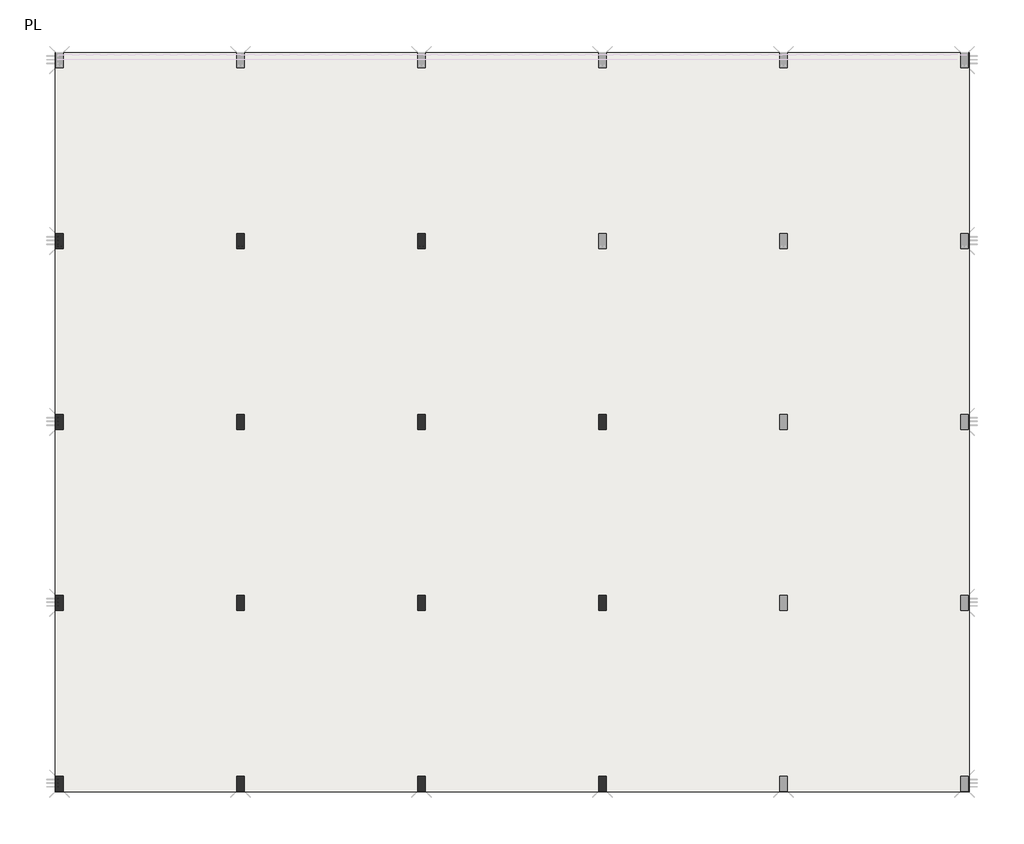
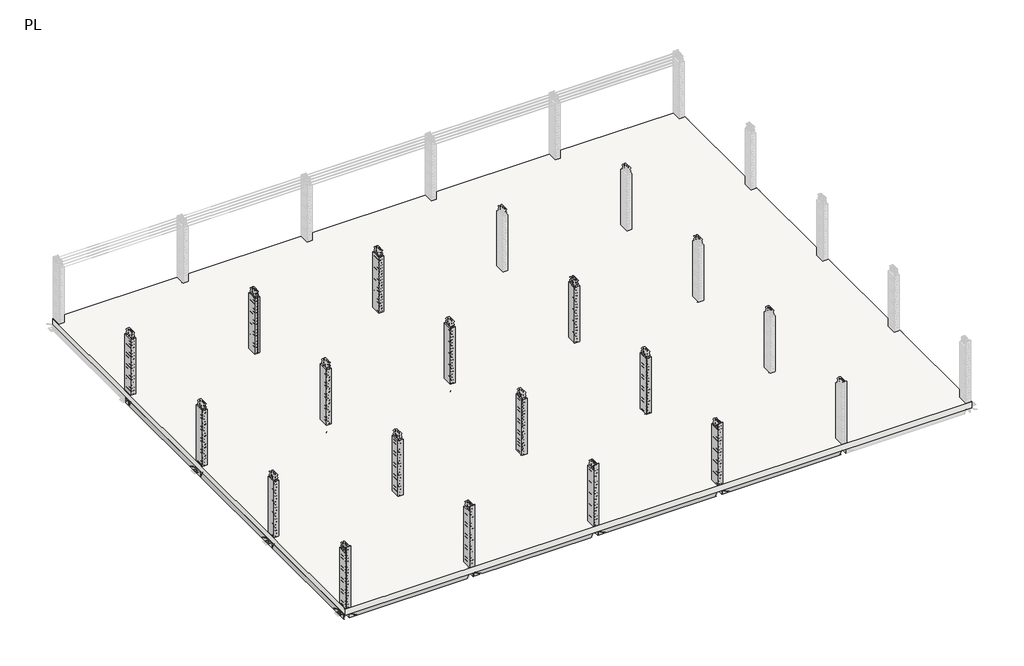
# One storey, part 1 of 10: 25 beams, 15 columns, 1 slab.
"""IFC4 building model written with IfcOpenShell, lengths in millimetres."""

from ifc_helpers import new_model, si_unit, frame, origin, place, context, project, spatial, polyline, outline, extrude, faceted_brep, element, save

model = new_model("IFC4")

# Units and contexts
model_context = context("Model", 3, world=origin())
ifc_project = project(units=[si_unit("LENGTHUNIT", "METRE", prefix="MILLI")], contexts=[model_context])

# Site, building, storey
site = spatial("IfcSite", under=ifc_project)
building = spatial("IfcBuilding", under=site)
storey = spatial("IfcBuildingStorey", under=building, Name="PL", Elevation=271.0)

# Beams
placement = place(None, origin())
element("IfcBeam", 1, ObjectType="Concrete-Rectangular Beam : 300 x 600mm", at=placement, inside=storey, context=model_context, shape_type="Brep", body=[
    faceted_brep([(-16585.9544379, -20429.1167521, -329.0), (-16560.9544379, -20429.1167521, -329.0), (-16560.9544379, -20429.1167521, -29.0), (-16585.9544379, -20429.1167521, -29.0), (-16560.9544379, -20129.1167521, -329.0), (-16585.9544379, -20129.1167521, -329.0), (-16585.9544379, -20129.1167521, -29.0), (-16560.9544379, -20129.1167521, -29.0)], [[[0, 1, 2, 3]], [[4, 1, 0, 5]], [[4, 5, 6, 7]], [[1, 4, 7, 2]], [[5, 0, 3, 6]], [[3, 2, 7, 6]]]),
    faceted_brep([(-22956.9544379, -20129.1167521, -329.0), (-22956.9544379, -20429.1167521, -329.0), (-22956.9544379, -20429.1167521, -29.0), (-22956.9544379, -20129.1167521, -29.0), (-22931.9544379, -20429.1167521, -329.0), (-22931.9544379, -20129.1167521, -329.0), (-22931.9544379, -20129.1167521, -29.0), (-22931.9544379, -20429.1167521, -29.0)], [[[0, 1, 2, 3]], [[4, 5, 6, 7]], [[1, 4, 7, 2]], [[1, 0, 5, 4]], [[5, 0, 3, 6]], [[3, 2, 7, 6]]]),
    faceted_brep([(-22681.9544379, -20129.1167521, -329.0), (-22681.9544379, -20429.1167521, -329.0), (-22681.9544379, -20429.1167521, -29.0), (-22681.9544379, -20129.1167521, -29.0), (-16835.9544379, -20429.1167521, -329.0), (-16835.9544379, -20129.1167521, -329.0), (-16835.9544379, -20129.1167521, -29.0), (-16835.9544379, -20429.1167521, -29.0), (-22656.9544379, -20129.1167521, -329.0), (-16860.9544379, -20129.1167521, -329.0), (-22656.9544379, -20129.1167521, -29.0), (-16860.9544379, -20129.1167521, -29.0)], [[[0, 1, 2, 3]], [[4, 5, 6, 7]], [[1, 4, 7, 2]], [[1, 0, 8, 9, 5, 4]], [[5, 9, 8, 0, 3, 10, 11, 6]], [[3, 2, 7, 6, 11, 10]]]),
])
element("IfcBeam", 2, ObjectType="Concrete-Rectangular Beam : 300 x 600mm", at=placement, inside=storey, context=model_context, shape_type="Brep", body=[
    faceted_brep([(-10489.9544379, -20429.1167521, -329.0), (-10464.9544379, -20429.1167521, -329.0), (-10464.9544379, -20429.1167521, -29.0), (-10489.9544379, -20429.1167521, -29.0), (-10464.9544379, -20129.1167521, -329.0), (-10489.9544379, -20129.1167521, -329.0), (-10489.9544379, -20129.1167521, -29.0), (-10464.9544379, -20129.1167521, -29.0)], [[[0, 1, 2, 3]], [[4, 1, 0, 5]], [[4, 5, 6, 7]], [[1, 4, 7, 2]], [[5, 0, 3, 6]], [[3, 2, 7, 6]]]),
    faceted_brep([(-16560.9544379, -20129.1167521, -329.0), (-16560.9544379, -20429.1167521, -329.0), (-16560.9544379, -20429.1167521, -29.0), (-16560.9544379, -20129.1167521, -29.0), (-10739.9544379, -20429.1167521, -329.0), (-10739.9544379, -20129.1167521, -329.0), (-10739.9544379, -20129.1167521, -29.0), (-10739.9544379, -20429.1167521, -29.0), (-10764.9544379, -20129.1167521, -329.0), (-10764.9544379, -20129.1167521, -29.0)], [[[0, 1, 2, 3]], [[4, 5, 6, 7]], [[1, 4, 7, 2]], [[1, 0, 8, 5, 4]], [[5, 8, 0, 3, 9, 6]], [[3, 2, 7, 6, 9]]]),
])
element("IfcBeam", 3, ObjectType="Concrete-Rectangular Beam : 300 x 600mm", at=placement, inside=storey, context=model_context, shape_type="Brep", body=[
    faceted_brep([(-4393.9544379, -20429.1167521, -329.0), (-4368.9544379, -20429.1167521, -329.0), (-4368.9544379, -20429.1167521, -29.0), (-4393.9544379, -20429.1167521, -29.0), (-4368.9544379, -20129.1167521, -329.0), (-4393.9544379, -20129.1167521, -329.0), (-4393.9544379, -20129.1167521, -29.0), (-4368.9544379, -20129.1167521, -29.0)], [[[0, 1, 2, 3]], [[4, 1, 0, 5]], [[4, 5, 6, 7]], [[1, 4, 7, 2]], [[5, 0, 3, 6]], [[3, 2, 7, 6]]]),
    faceted_brep([(-10464.9544379, -20129.1167521, -329.0), (-10464.9544379, -20429.1167521, -329.0), (-10464.9544379, -20429.1167521, -29.0), (-10464.9544379, -20129.1167521, -29.0), (-4643.9544379, -20429.1167521, -329.0), (-4643.9544379, -20129.1167521, -329.0), (-4643.9544379, -20129.1167521, -29.0), (-4643.9544379, -20429.1167521, -29.0), (-4668.9544379, -20129.1167521, -329.0), (-4668.9544379, -20129.1167521, -29.0)], [[[0, 1, 2, 3]], [[4, 5, 6, 7]], [[1, 4, 7, 2]], [[1, 0, 8, 5, 4]], [[5, 8, 0, 3, 9, 6]], [[3, 2, 7, 6, 9]]]),
])
element("IfcBeam", 4, ObjectType="Concrete-Rectangular Beam : 300 x 600mm", at=placement, inside=storey, context=model_context, shape_type="Brep", body=[
    faceted_brep([(1702.0455621, -20429.1167521, -329.0), (1727.0455621, -20429.1167521, -329.0), (1727.0455621, -20429.1167521, -29.0), (1702.0455621, -20429.1167521, -29.0), (1727.0455621, -20129.1167521, -329.0), (1702.0455621, -20129.1167521, -329.0), (1702.0455621, -20129.1167521, -29.0), (1727.0455621, -20129.1167521, -29.0)], [[[0, 1, 2, 3]], [[4, 1, 0, 5]], [[4, 5, 6, 7]], [[1, 4, 7, 2]], [[5, 0, 3, 6]], [[3, 2, 7, 6]]]),
    faceted_brep([(-4368.9544379, -20129.1167521, -329.0), (-4368.9544379, -20429.1167521, -329.0), (-4368.9544379, -20429.1167521, -29.0), (-4368.9544379, -20129.1167521, -29.0), (1452.0455621, -20429.1167521, -329.0), (1452.0455621, -20129.1167521, -329.0), (1452.0455621, -20129.1167521, -29.0), (1452.0455621, -20429.1167521, -29.0), (1427.0455621, -20129.1167521, -329.0), (1427.0455621, -20129.1167521, -29.0)], [[[0, 1, 2, 3]], [[4, 5, 6, 7]], [[1, 4, 7, 2]], [[1, 0, 8, 5, 4]], [[5, 8, 0, 3, 9, 6]], [[3, 2, 7, 6, 9]]]),
])
element("IfcBeam", 5, ObjectType="Concrete-Rectangular Beam : 300 x 600mm", at=placement, inside=storey, context=model_context, shape_type="Brep", body=[
    faceted_brep([(-16585.9544379, -14333.1167521, -329.0), (-16560.9544379, -14333.1167521, -329.0), (-16560.9544379, -14333.1167521, -29.0), (-16585.9544379, -14333.1167521, -29.0), (-16560.9544379, -14033.1167521, -329.0), (-16585.9544379, -14033.1167521, -329.0), (-16585.9544379, -14033.1167521, -29.0), (-16560.9544379, -14033.1167521, -29.0)], [[[0, 1, 2, 3]], [[4, 1, 0, 5]], [[4, 5, 6, 7]], [[1, 4, 7, 2]], [[5, 0, 3, 6]], [[3, 2, 7, 6]]]),
    faceted_brep([(-22956.9544379, -14033.1167521, -329.0), (-22956.9544379, -14333.1167521, -329.0), (-22956.9544379, -14333.1167521, -29.0), (-22956.9544379, -14033.1167521, -29.0), (-22931.9544379, -14333.1167521, -329.0), (-22931.9544379, -14033.1167521, -329.0), (-22931.9544379, -14033.1167521, -29.0), (-22931.9544379, -14333.1167521, -29.0)], [[[0, 1, 2, 3]], [[4, 5, 6, 7]], [[1, 4, 7, 2]], [[1, 0, 5, 4]], [[5, 0, 3, 6]], [[3, 2, 7, 6]]]),
    faceted_brep([(-22681.9544379, -14033.1167521, -329.0), (-22681.9544379, -14333.1167521, -329.0), (-22681.9544379, -14333.1167521, -29.0), (-22681.9544379, -14033.1167521, -29.0), (-16835.9544379, -14333.1167521, -329.0), (-16835.9544379, -14033.1167521, -329.0), (-16835.9544379, -14033.1167521, -29.0), (-16835.9544379, -14333.1167521, -29.0), (-22656.9544379, -14333.1167521, -329.0), (-16860.9544379, -14333.1167521, -329.0), (-16860.9544379, -14333.1167521, -29.0), (-22656.9544379, -14333.1167521, -29.0), (-22656.9544379, -14033.1167521, -329.0), (-16860.9544379, -14033.1167521, -329.0), (-22656.9544379, -14033.1167521, -29.0), (-16860.9544379, -14033.1167521, -29.0)], [[[0, 1, 2, 3]], [[4, 5, 6, 7]], [[1, 8, 9, 4, 7, 10, 11, 2]], [[1, 0, 12, 13, 5, 4, 9, 8]], [[5, 13, 12, 0, 3, 14, 15, 6]], [[3, 2, 11, 10, 7, 6, 15, 14]]]),
])
element("IfcBeam", 6, ObjectType="Concrete-Rectangular Beam : 300 x 600mm", at=placement, inside=storey, context=model_context, shape_type="Brep", body=[
    faceted_brep([(-10489.9544379, -14333.1167521, -329.0), (-10464.9544379, -14333.1167521, -329.0), (-10464.9544379, -14333.1167521, -29.0), (-10489.9544379, -14333.1167521, -29.0), (-10464.9544379, -14033.1167521, -329.0), (-10489.9544379, -14033.1167521, -329.0), (-10489.9544379, -14033.1167521, -29.0), (-10464.9544379, -14033.1167521, -29.0)], [[[0, 1, 2, 3]], [[4, 1, 0, 5]], [[4, 5, 6, 7]], [[1, 4, 7, 2]], [[5, 0, 3, 6]], [[3, 2, 7, 6]]]),
    faceted_brep([(-16560.9544379, -14033.1167521, -329.0), (-16560.9544379, -14333.1167521, -329.0), (-16560.9544379, -14333.1167521, -29.0), (-16560.9544379, -14033.1167521, -29.0), (-10739.9544379, -14333.1167521, -329.0), (-10739.9544379, -14033.1167521, -329.0), (-10739.9544379, -14033.1167521, -29.0), (-10739.9544379, -14333.1167521, -29.0), (-10764.9544379, -14333.1167521, -329.0), (-10764.9544379, -14333.1167521, -29.0), (-10764.9544379, -14033.1167521, -329.0), (-10764.9544379, -14033.1167521, -29.0)], [[[0, 1, 2, 3]], [[4, 5, 6, 7]], [[1, 8, 4, 7, 9, 2]], [[1, 0, 10, 5, 4, 8]], [[5, 10, 0, 3, 11, 6]], [[3, 2, 9, 7, 6, 11]]]),
])
element("IfcBeam", 7, ObjectType="Concrete-Rectangular Beam : 300 x 600mm", at=placement, inside=storey, context=model_context, shape_type="Brep", body=[
    faceted_brep([(-4393.9544379, -14333.1167521, -329.0), (-4368.9544379, -14333.1167521, -329.0), (-4368.9544379, -14333.1167521, -29.0), (-4393.9544379, -14333.1167521, -29.0), (-4368.9544379, -14033.1167521, -329.0), (-4393.9544379, -14033.1167521, -329.0), (-4393.9544379, -14033.1167521, -29.0), (-4368.9544379, -14033.1167521, -29.0)], [[[0, 1, 2, 3]], [[4, 1, 0, 5]], [[4, 5, 6, 7]], [[1, 4, 7, 2]], [[5, 0, 3, 6]], [[3, 2, 7, 6]]]),
    faceted_brep([(-10464.9544379, -14033.1167521, -329.0), (-10464.9544379, -14333.1167521, -329.0), (-10464.9544379, -14333.1167521, -29.0), (-10464.9544379, -14033.1167521, -29.0), (-4643.9544379, -14333.1167521, -329.0), (-4643.9544379, -14033.1167521, -329.0), (-4643.9544379, -14033.1167521, -29.0), (-4643.9544379, -14333.1167521, -29.0), (-4668.9544379, -14333.1167521, -329.0), (-4668.9544379, -14333.1167521, -29.0), (-4668.9544379, -14033.1167521, -329.0), (-4668.9544379, -14033.1167521, -29.0)], [[[0, 1, 2, 3]], [[4, 5, 6, 7]], [[1, 8, 4, 7, 9, 2]], [[1, 0, 10, 5, 4, 8]], [[5, 10, 0, 3, 11, 6]], [[3, 2, 9, 7, 6, 11]]]),
])
element("IfcBeam", 8, ObjectType="Concrete-Rectangular Beam : 300 x 600mm", at=placement, inside=storey, context=model_context, shape_type="Brep", body=[
    faceted_brep([(1702.0455621, -14333.1167521, -329.0), (1727.0455621, -14333.1167521, -329.0), (1727.0455621, -14333.1167521, -29.0), (1702.0455621, -14333.1167521, -29.0), (1727.0455621, -14033.1167521, -329.0), (1702.0455621, -14033.1167521, -329.0), (1702.0455621, -14033.1167521, -29.0), (1727.0455621, -14033.1167521, -29.0)], [[[0, 1, 2, 3]], [[4, 1, 0, 5]], [[4, 5, 6, 7]], [[1, 4, 7, 2]], [[5, 0, 3, 6]], [[3, 2, 7, 6]]]),
    faceted_brep([(-4368.9544379, -14033.1167521, -329.0), (-4368.9544379, -14333.1167521, -329.0), (-4368.9544379, -14333.1167521, -29.0), (-4368.9544379, -14033.1167521, -29.0), (1452.0455621, -14333.1167521, -329.0), (1452.0455621, -14033.1167521, -329.0), (1452.0455621, -14033.1167521, -29.0), (1452.0455621, -14333.1167521, -29.0), (1427.0455621, -14333.1167521, -329.0), (1427.0455621, -14333.1167521, -29.0), (1427.0455621, -14033.1167521, -329.0), (1427.0455621, -14033.1167521, -29.0)], [[[0, 1, 2, 3]], [[4, 5, 6, 7]], [[1, 8, 4, 7, 9, 2]], [[1, 0, 10, 5, 4, 8]], [[5, 10, 0, 3, 11, 6]], [[3, 2, 9, 7, 6, 11]]]),
])
element("IfcBeam", 9, ObjectType="Concrete-Rectangular Beam : 300 x 600mm", at=placement, inside=storey, context=model_context, shape_type="Brep", body=[
    faceted_brep([(-16585.9544379, -8237.1167521, -329.0), (-16560.9544379, -8237.1167521, -329.0), (-16560.9544379, -8237.1167521, -29.0), (-16585.9544379, -8237.1167521, -29.0), (-16560.9544379, -7937.1167521, -329.0), (-16585.9544379, -7937.1167521, -329.0), (-16585.9544379, -7937.1167521, -29.0), (-16560.9544379, -7937.1167521, -29.0)], [[[0, 1, 2, 3]], [[4, 1, 0, 5]], [[4, 5, 6, 7]], [[1, 4, 7, 2]], [[5, 0, 3, 6]], [[3, 2, 7, 6]]]),
    faceted_brep([(-22956.9544379, -7937.1167521, -329.0), (-22956.9544379, -8237.1167521, -329.0), (-22956.9544379, -8237.1167521, -29.0), (-22956.9544379, -7937.1167521, -29.0), (-22931.9544379, -8237.1167521, -329.0), (-22931.9544379, -7937.1167521, -329.0), (-22931.9544379, -7937.1167521, -29.0), (-22931.9544379, -8237.1167521, -29.0)], [[[0, 1, 2, 3]], [[4, 5, 6, 7]], [[1, 4, 7, 2]], [[1, 0, 5, 4]], [[5, 0, 3, 6]], [[3, 2, 7, 6]]]),
    faceted_brep([(-22681.9544379, -7937.1167521, -329.0), (-22681.9544379, -8237.1167521, -329.0), (-22681.9544379, -8237.1167521, -29.0), (-22681.9544379, -7937.1167521, -29.0), (-16835.9544379, -8237.1167521, -329.0), (-16835.9544379, -7937.1167521, -329.0), (-16835.9544379, -7937.1167521, -29.0), (-16835.9544379, -8237.1167521, -29.0), (-22656.9544379, -8237.1167521, -329.0), (-16860.9544379, -8237.1167521, -329.0), (-16860.9544379, -8237.1167521, -29.0), (-22656.9544379, -8237.1167521, -29.0), (-22656.9544379, -7937.1167521, -329.0), (-16860.9544379, -7937.1167521, -329.0), (-22656.9544379, -7937.1167521, -29.0), (-16860.9544379, -7937.1167521, -29.0)], [[[0, 1, 2, 3]], [[4, 5, 6, 7]], [[1, 8, 9, 4, 7, 10, 11, 2]], [[1, 0, 12, 13, 5, 4, 9, 8]], [[5, 13, 12, 0, 3, 14, 15, 6]], [[3, 2, 11, 10, 7, 6, 15, 14]]]),
])
element("IfcBeam", 10, ObjectType="Concrete-Rectangular Beam : 300 x 600mm", at=placement, inside=storey, context=model_context, shape_type="Brep", body=[
    faceted_brep([(-10489.9544379, -8237.1167521, -329.0), (-10464.9544379, -8237.1167521, -329.0), (-10464.9544379, -8237.1167521, -29.0), (-10489.9544379, -8237.1167521, -29.0), (-10464.9544379, -7937.1167521, -329.0), (-10489.9544379, -7937.1167521, -329.0), (-10489.9544379, -7937.1167521, -29.0), (-10464.9544379, -7937.1167521, -29.0)], [[[0, 1, 2, 3]], [[4, 1, 0, 5]], [[4, 5, 6, 7]], [[1, 4, 7, 2]], [[5, 0, 3, 6]], [[3, 2, 7, 6]]]),
    faceted_brep([(-16560.9544379, -7937.1167521, -329.0), (-16560.9544379, -8237.1167521, -329.0), (-16560.9544379, -8237.1167521, -29.0), (-16560.9544379, -7937.1167521, -29.0), (-10739.9544379, -8237.1167521, -329.0), (-10739.9544379, -7937.1167521, -329.0), (-10739.9544379, -7937.1167521, -29.0), (-10739.9544379, -8237.1167521, -29.0), (-10764.9544379, -8237.1167521, -329.0), (-10764.9544379, -8237.1167521, -29.0), (-10764.9544379, -7937.1167521, -329.0), (-10764.9544379, -7937.1167521, -29.0)], [[[0, 1, 2, 3]], [[4, 5, 6, 7]], [[1, 8, 4, 7, 9, 2]], [[1, 0, 10, 5, 4, 8]], [[5, 10, 0, 3, 11, 6]], [[3, 2, 9, 7, 6, 11]]]),
])
element("IfcBeam", 11, ObjectType="Concrete-Rectangular Beam : 300 x 600mm", at=placement, inside=storey, context=model_context, shape_type="Brep", body=[
    faceted_brep([(-4393.9544379, -8237.1167521, -329.0), (-4368.9544379, -8237.1167521, -329.0), (-4368.9544379, -8237.1167521, -29.0), (-4393.9544379, -8237.1167521, -29.0), (-4368.9544379, -7937.1167521, -329.0), (-4393.9544379, -7937.1167521, -329.0), (-4393.9544379, -7937.1167521, -29.0), (-4368.9544379, -7937.1167521, -29.0)], [[[0, 1, 2, 3]], [[4, 1, 0, 5]], [[4, 5, 6, 7]], [[1, 4, 7, 2]], [[5, 0, 3, 6]], [[3, 2, 7, 6]]]),
    faceted_brep([(-10464.9544379, -7937.1167521, -329.0), (-10464.9544379, -8237.1167521, -329.0), (-10464.9544379, -8237.1167521, -29.0), (-10464.9544379, -7937.1167521, -29.0), (-4643.9544379, -8237.1167521, -329.0), (-4643.9544379, -7937.1167521, -329.0), (-4643.9544379, -7937.1167521, -29.0), (-4643.9544379, -8237.1167521, -29.0), (-4668.9544379, -8237.1167521, -329.0), (-4668.9544379, -8237.1167521, -29.0), (-4668.9544379, -7937.1167521, -329.0), (-4668.9544379, -7937.1167521, -29.0)], [[[0, 1, 2, 3]], [[4, 5, 6, 7]], [[1, 8, 4, 7, 9, 2]], [[1, 0, 10, 5, 4, 8]], [[5, 10, 0, 3, 11, 6]], [[3, 2, 9, 7, 6, 11]]]),
])
element("IfcBeam", 12, ObjectType="Concrete-Rectangular Beam : 300 x 600mm", at=placement, inside=storey, context=model_context, shape_type="Brep", body=[
    faceted_brep([(1702.0455621, -8237.1167521, -329.0), (1727.0455621, -8237.1167521, -329.0), (1727.0455621, -8237.1167521, -29.0), (1702.0455621, -8237.1167521, -29.0), (1727.0455621, -7937.1167521, -329.0), (1702.0455621, -7937.1167521, -329.0), (1702.0455621, -7937.1167521, -29.0), (1727.0455621, -7937.1167521, -29.0)], [[[0, 1, 2, 3]], [[4, 1, 0, 5]], [[4, 5, 6, 7]], [[1, 4, 7, 2]], [[5, 0, 3, 6]], [[3, 2, 7, 6]]]),
    faceted_brep([(-4368.9544379, -7937.1167521, -329.0), (-4368.9544379, -8237.1167521, -329.0), (-4368.9544379, -8237.1167521, -29.0), (-4368.9544379, -7937.1167521, -29.0), (1452.0455621, -8237.1167521, -329.0), (1452.0455621, -7937.1167521, -329.0), (1452.0455621, -7937.1167521, -29.0), (1452.0455621, -8237.1167521, -29.0), (1427.0455621, -8237.1167521, -329.0), (1427.0455621, -8237.1167521, -29.0), (1427.0455621, -7937.1167521, -329.0), (1427.0455621, -7937.1167521, -29.0)], [[[0, 1, 2, 3]], [[4, 5, 6, 7]], [[1, 8, 4, 7, 9, 2]], [[1, 0, 10, 5, 4, 8]], [[5, 10, 0, 3, 11, 6]], [[3, 2, 9, 7, 6, 11]]]),
])
element("IfcBeam", 13, ObjectType="Concrete-Rectangular Beam : 300 x 600mm", at=placement, inside=storey, context=model_context, shape_type="Brep", body=[
    faceted_brep([(-16585.9544379, -2141.1167521, -329.0), (-16560.9544379, -2141.1167521, -329.0), (-16560.9544379, -2141.1167521, -29.0), (-16585.9544379, -2141.1167521, -29.0), (-16560.9544379, -1841.1167521, -329.0), (-16585.9544379, -1841.1167521, -329.0), (-16585.9544379, -1841.1167521, -29.0), (-16560.9544379, -1841.1167521, -29.0)], [[[0, 1, 2, 3]], [[4, 1, 0, 5]], [[4, 5, 6, 7]], [[1, 4, 7, 2]], [[5, 0, 3, 6]], [[3, 2, 7, 6]]]),
    faceted_brep([(-22956.9544379, -1841.1167521, -329.0), (-22956.9544379, -2141.1167521, -329.0), (-22956.9544379, -2141.1167521, -29.0), (-22956.9544379, -1841.1167521, -29.0), (-22931.9544379, -2141.1167521, -329.0), (-22931.9544379, -1841.1167521, -329.0), (-22931.9544379, -1841.1167521, -29.0), (-22931.9544379, -2141.1167521, -29.0)], [[[0, 1, 2, 3]], [[4, 5, 6, 7]], [[1, 4, 7, 2]], [[1, 0, 5, 4]], [[5, 0, 3, 6]], [[3, 2, 7, 6]]]),
    faceted_brep([(-22681.9544379, -1841.1167521, -329.0), (-22681.9544379, -2141.1167521, -329.0), (-22681.9544379, -2141.1167521, -29.0), (-22681.9544379, -1841.1167521, -29.0), (-16835.9544379, -2141.1167521, -329.0), (-16835.9544379, -1841.1167521, -329.0), (-16835.9544379, -1841.1167521, -29.0), (-16835.9544379, -2141.1167521, -29.0), (-22656.9544379, -2141.1167521, -329.0), (-16860.9544379, -2141.1167521, -329.0), (-16860.9544379, -2141.1167521, -29.0), (-22656.9544379, -2141.1167521, -29.0), (-22656.9544379, -1841.1167521, -329.0), (-16860.9544379, -1841.1167521, -329.0), (-22656.9544379, -1841.1167521, -29.0), (-16860.9544379, -1841.1167521, -29.0)], [[[0, 1, 2, 3]], [[4, 5, 6, 7]], [[1, 8, 9, 4, 7, 10, 11, 2]], [[1, 0, 12, 13, 5, 4, 9, 8]], [[5, 13, 12, 0, 3, 14, 15, 6]], [[3, 2, 11, 10, 7, 6, 15, 14]]]),
])
element("IfcBeam", 14, ObjectType="Concrete-Rectangular Beam : 300 x 600mm", at=placement, inside=storey, context=model_context, shape_type="Brep", body=[
    faceted_brep([(-10489.9544379, -2141.1167521, -329.0), (-10464.9544379, -2141.1167521, -329.0), (-10464.9544379, -2141.1167521, -29.0), (-10489.9544379, -2141.1167521, -29.0), (-10464.9544379, -1841.1167521, -329.0), (-10489.9544379, -1841.1167521, -329.0), (-10489.9544379, -1841.1167521, -29.0), (-10464.9544379, -1841.1167521, -29.0)], [[[0, 1, 2, 3]], [[4, 1, 0, 5]], [[4, 5, 6, 7]], [[1, 4, 7, 2]], [[5, 0, 3, 6]], [[3, 2, 7, 6]]]),
    faceted_brep([(-16560.9544379, -1841.1167521, -329.0), (-16560.9544379, -2141.1167521, -329.0), (-16560.9544379, -2141.1167521, -29.0), (-16560.9544379, -1841.1167521, -29.0), (-10739.9544379, -2141.1167521, -329.0), (-10739.9544379, -1841.1167521, -329.0), (-10739.9544379, -1841.1167521, -29.0), (-10739.9544379, -2141.1167521, -29.0), (-10764.9544379, -2141.1167521, -329.0), (-10764.9544379, -2141.1167521, -29.0), (-10764.9544379, -1841.1167521, -329.0), (-10764.9544379, -1841.1167521, -29.0)], [[[0, 1, 2, 3]], [[4, 5, 6, 7]], [[1, 8, 4, 7, 9, 2]], [[1, 0, 10, 5, 4, 8]], [[5, 10, 0, 3, 11, 6]], [[3, 2, 9, 7, 6, 11]]]),
])
element("IfcBeam", 15, ObjectType="Concrete-Rectangular Beam : 300 x 600mm", at=placement, inside=storey, context=model_context, shape_type="SweptSolid", body=[
    extrude(outline(polyline([(-22931.9544379, -20129.1167521), (-22956.9544379, -20129.1167521), (-22956.9544379, -14333.1167521), (-22931.9544379, -14333.1167521), (-22931.9544379, -14433.1167521), (-22681.9544379, -14433.1167521), (-22681.9544379, -14333.1167521), (-22656.9544379, -14333.1167521), (-22656.9544379, -20129.1167521), (-22681.9544379, -20129.1167521), (-22681.9544379, -20029.1167521), (-22931.9544379, -20029.1167521), (-22931.9544379, -20129.1167521)])), frame((0.0, 0.0, -329.0), z_axis=(0.0, 0.0, 1.0), x_axis=(1.0, 0.0, 0.0)), (0.0, 0.0, 1.0), 300.0),
])
element("IfcBeam", 16, ObjectType="Concrete-Rectangular Beam : 300 x 600mm", at=placement, inside=storey, context=model_context, shape_type="SweptSolid", body=[
    extrude(outline(polyline([(-22931.9544379, -14033.1167521), (-22956.9544379, -14033.1167521), (-22956.9544379, -8237.1167521), (-22931.9544379, -8237.1167521), (-22931.9544379, -8337.1167521), (-22681.9544379, -8337.1167521), (-22681.9544379, -8237.1167521), (-22656.9544379, -8237.1167521), (-22656.9544379, -14033.1167521), (-22681.9544379, -14033.1167521), (-22681.9544379, -13933.1167521), (-22931.9544379, -13933.1167521), (-22931.9544379, -14033.1167521)])), frame((0.0, 0.0, -329.0), z_axis=(0.0, 0.0, 1.0), x_axis=(1.0, 0.0, 0.0)), (0.0, 0.0, 1.0), 300.0),
])
element("IfcBeam", 17, ObjectType="Concrete-Rectangular Beam : 300 x 600mm", at=placement, inside=storey, context=model_context, shape_type="SweptSolid", body=[
    extrude(outline(polyline([(-22931.9544379, -7937.1167521), (-22956.9544379, -7937.1167521), (-22956.9544379, -2141.1167521), (-22931.9544379, -2141.1167521), (-22931.9544379, -2241.1167521), (-22681.9544379, -2241.1167521), (-22681.9544379, -2141.1167521), (-22656.9544379, -2141.1167521), (-22656.9544379, -7937.1167521), (-22681.9544379, -7937.1167521), (-22681.9544379, -7837.1167521), (-22931.9544379, -7837.1167521), (-22931.9544379, -7937.1167521)])), frame((0.0, 0.0, -329.0), z_axis=(0.0, 0.0, 1.0), x_axis=(1.0, 0.0, 0.0)), (0.0, 0.0, 1.0), 300.0),
])
element("IfcBeam", 18, ObjectType="Concrete-Rectangular Beam : 300 x 600mm", at=placement, inside=storey, context=model_context, shape_type="SweptSolid", body=[
    extrude(outline(polyline([(-16835.9544379, -20129.1167521), (-16860.9544379, -20129.1167521), (-16860.9544379, -14333.1167521), (-16835.9544379, -14333.1167521), (-16835.9544379, -14433.1167521), (-16585.9544379, -14433.1167521), (-16585.9544379, -14333.1167521), (-16560.9544379, -14333.1167521), (-16560.9544379, -20129.1167521), (-16585.9544379, -20129.1167521), (-16585.9544379, -20029.1167521), (-16835.9544379, -20029.1167521), (-16835.9544379, -20129.1167521)])), frame((0.0, 0.0, -329.0), z_axis=(0.0, 0.0, 1.0), x_axis=(1.0, 0.0, 0.0)), (0.0, 0.0, 1.0), 300.0),
])
element("IfcBeam", 19, ObjectType="Concrete-Rectangular Beam : 300 x 600mm", at=placement, inside=storey, context=model_context, shape_type="SweptSolid", body=[
    extrude(outline(polyline([(-16835.9544379, -14033.1167521), (-16860.9544379, -14033.1167521), (-16860.9544379, -8237.1167521), (-16835.9544379, -8237.1167521), (-16835.9544379, -8337.1167521), (-16585.9544379, -8337.1167521), (-16585.9544379, -8237.1167521), (-16560.9544379, -8237.1167521), (-16560.9544379, -14033.1167521), (-16585.9544379, -14033.1167521), (-16585.9544379, -13933.1167521), (-16835.9544379, -13933.1167521), (-16835.9544379, -14033.1167521)])), frame((0.0, 0.0, -329.0), z_axis=(0.0, 0.0, 1.0), x_axis=(1.0, 0.0, 0.0)), (0.0, 0.0, 1.0), 300.0),
])
element("IfcBeam", 20, ObjectType="Concrete-Rectangular Beam : 300 x 600mm", at=placement, inside=storey, context=model_context, shape_type="SweptSolid", body=[
    extrude(outline(polyline([(-16835.9544379, -7937.1167521), (-16860.9544379, -7937.1167521), (-16860.9544379, -2141.1167521), (-16835.9544379, -2141.1167521), (-16835.9544379, -2241.1167521), (-16585.9544379, -2241.1167521), (-16585.9544379, -2141.1167521), (-16560.9544379, -2141.1167521), (-16560.9544379, -7937.1167521), (-16585.9544379, -7937.1167521), (-16585.9544379, -7837.1167521), (-16835.9544379, -7837.1167521), (-16835.9544379, -7937.1167521)])), frame((0.0, 0.0, -329.0), z_axis=(0.0, 0.0, 1.0), x_axis=(1.0, 0.0, 0.0)), (0.0, 0.0, 1.0), 300.0),
])
element("IfcBeam", 21, ObjectType="Concrete-Rectangular Beam : 300 x 600mm", at=placement, inside=storey, context=model_context, shape_type="SweptSolid", body=[
    extrude(outline(polyline([(-10739.9544379, -20129.1167521), (-10764.9544379, -20129.1167521), (-10764.9544379, -14333.1167521), (-10739.9544379, -14333.1167521), (-10739.9544379, -14433.1167521), (-10489.9544379, -14433.1167521), (-10489.9544379, -14333.1167521), (-10464.9544379, -14333.1167521), (-10464.9544379, -20129.1167521), (-10489.9544379, -20129.1167521), (-10489.9544379, -20029.1167521), (-10739.9544379, -20029.1167521), (-10739.9544379, -20129.1167521)])), frame((0.0, 0.0, -329.0), z_axis=(0.0, 0.0, 1.0), x_axis=(1.0, 0.0, 0.0)), (0.0, 0.0, 1.0), 300.0),
])
element("IfcBeam", 22, ObjectType="Concrete-Rectangular Beam : 300 x 600mm", at=placement, inside=storey, context=model_context, shape_type="SweptSolid", body=[
    extrude(outline(polyline([(-10739.9544379, -14033.1167521), (-10764.9544379, -14033.1167521), (-10764.9544379, -8237.1167521), (-10739.9544379, -8237.1167521), (-10739.9544379, -8337.1167521), (-10489.9544379, -8337.1167521), (-10489.9544379, -8237.1167521), (-10464.9544379, -8237.1167521), (-10464.9544379, -14033.1167521), (-10489.9544379, -14033.1167521), (-10489.9544379, -13933.1167521), (-10739.9544379, -13933.1167521), (-10739.9544379, -14033.1167521)])), frame((0.0, 0.0, -329.0), z_axis=(0.0, 0.0, 1.0), x_axis=(1.0, 0.0, 0.0)), (0.0, 0.0, 1.0), 300.0),
])
element("IfcBeam", 23, ObjectType="Concrete-Rectangular Beam : 300 x 600mm", at=placement, inside=storey, context=model_context, shape_type="SweptSolid", body=[
    extrude(outline(polyline([(-10489.9544379, -7837.1167521), (-10739.9544379, -7837.1167521), (-10739.9544379, -7937.1167521), (-10764.9544379, -7937.1167521), (-10764.9544379, -2141.1167521), (-10739.9544379, -2141.1167521), (-10739.9544379, -2241.1167521), (-10489.9544379, -2241.1167521), (-10489.9544379, -2141.1167521), (-10464.9544379, -2141.1167521), (-10464.9544379, -7937.1167521), (-10489.9544379, -7937.1167521), (-10489.9544379, -7837.1167521)])), frame((0.0, 0.0, -329.0), z_axis=(0.0, 0.0, 1.0), x_axis=(1.0, 0.0, 0.0)), (0.0, 0.0, 1.0), 300.0),
])
element("IfcBeam", 24, ObjectType="Concrete-Rectangular Beam : 300 x 600mm", at=placement, inside=storey, context=model_context, shape_type="SweptSolid", body=[
    extrude(outline(polyline([(-4643.9544379, -20129.1167521), (-4668.9544379, -20129.1167521), (-4668.9544379, -14333.1167521), (-4643.9544379, -14333.1167521), (-4643.9544379, -14433.1167521), (-4393.9544379, -14433.1167521), (-4393.9544379, -14333.1167521), (-4368.9544379, -14333.1167521), (-4368.9544379, -20129.1167521), (-4393.9544379, -20129.1167521), (-4393.9544379, -20029.1167521), (-4643.9544379, -20029.1167521), (-4643.9544379, -20129.1167521)])), frame((0.0, 0.0, -329.0), z_axis=(0.0, 0.0, 1.0), x_axis=(1.0, 0.0, 0.0)), (0.0, 0.0, 1.0), 300.0),
])
element("IfcBeam", 25, ObjectType="Concrete-Rectangular Beam : 300 x 600mm", at=placement, inside=storey, context=model_context, shape_type="SweptSolid", body=[
    extrude(outline(polyline([(-4643.9544379, -14033.1167521), (-4668.9544379, -14033.1167521), (-4668.9544379, -8237.1167521), (-4643.9544379, -8237.1167521), (-4643.9544379, -8337.1167521), (-4393.9544379, -8337.1167521), (-4393.9544379, -8237.1167521), (-4368.9544379, -8237.1167521), (-4368.9544379, -14033.1167521), (-4393.9544379, -14033.1167521), (-4393.9544379, -13933.1167521), (-4643.9544379, -13933.1167521), (-4643.9544379, -14033.1167521)])), frame((0.0, 0.0, -329.0), z_axis=(0.0, 0.0, 1.0), x_axis=(1.0, 0.0, 0.0)), (0.0, 0.0, 1.0), 300.0),
])

# Columns
element("IfcColumn", 26, ObjectType="Concrete-Rectangular-Column : 500X250", at=placement, inside=storey, context=model_context, shape_type="SweptSolid", body=[
    extrude(outline(polyline([(-20529.1167521, 271.0), (-20529.1167521, 3471.4), (-20525.9346398, 3471.4), (-20525.9346398, 3171.4), (-20029.1167521, 3171.4), (-20029.1167521, 271.0), (-20529.1167521, 271.0)])), frame((-22931.9544379, 0.0, 0.0), z_axis=(1.0, 0.0, 0.0), x_axis=(0.0, 1.0, 0.0)), (0.0, 0.0, 1.0), 250.0),
])
element("IfcColumn", 27, ObjectType="Concrete-Rectangular-Column : 500X250", at=placement, inside=storey, context=model_context, shape_type="SweptSolid", body=[
    extrude(outline(polyline([(-20529.1167521, 271.0), (-20529.1167521, 3471.4), (-20525.9346398, 3471.4), (-20525.9346398, 3171.4), (-20029.1167521, 3171.4), (-20029.1167521, 271.0), (-20529.1167521, 271.0)])), frame((-16835.9544379, 0.0, 0.0), z_axis=(1.0, 0.0, 0.0), x_axis=(0.0, 1.0, 0.0)), (0.0, 0.0, 1.0), 250.0),
])
element("IfcColumn", 28, ObjectType="Concrete-Rectangular-Column : 500X250", at=placement, inside=storey, context=model_context, shape_type="SweptSolid", body=[
    extrude(outline(polyline([(-20529.1167521, 271.0), (-20529.1167521, 3471.4), (-20525.9346398, 3471.4), (-20525.9346398, 3171.4), (-20029.1167521, 3171.4), (-20029.1167521, 271.0), (-20529.1167521, 271.0)])), frame((-10739.9544379, 0.0, 0.0), z_axis=(1.0, 0.0, 0.0), x_axis=(0.0, 1.0, 0.0)), (0.0, 0.0, 1.0), 250.0),
])
element("IfcColumn", 29, ObjectType="Concrete-Rectangular-Column : 500X250", at=placement, inside=storey, context=model_context, shape_type="SweptSolid", body=[
    extrude(outline(polyline([(-20529.1167521, 271.0), (-20529.1167521, 3471.4), (-20525.9346398, 3471.4), (-20525.9346398, 3171.4), (-20029.1167521, 3171.4), (-20029.1167521, 271.0), (-20529.1167521, 271.0)])), frame((-4643.9544379, 0.0, 0.0), z_axis=(1.0, 0.0, 0.0), x_axis=(0.0, 1.0, 0.0)), (0.0, 0.0, 1.0), 250.0),
])
element("IfcColumn", 30, ObjectType="Concrete-Rectangular-Column : 500X250", at=placement, inside=storey, context=model_context, shape_type="SweptSolid", body=[
    extrude(outline(polyline([(-22931.9544379, -13933.1167521), (-22681.9544379, -13933.1167521), (-22681.9544379, -14433.1167521), (-22931.9544379, -14433.1167521), (-22931.9544379, -13933.1167521)])), frame((0.0, 0.0, 271.0), z_axis=(0.0, 0.0, 1.0), x_axis=(1.0, 0.0, 0.0)), (0.0, 0.0, 1.0), 2900.4),
])
element("IfcColumn", 31, ObjectType="Concrete-Rectangular-Column : 500X250", at=placement, inside=storey, context=model_context, shape_type="SweptSolid", body=[
    extrude(outline(polyline([(-16835.9544379, -13933.1167521), (-16585.9544379, -13933.1167521), (-16585.9544379, -14433.1167521), (-16835.9544379, -14433.1167521), (-16835.9544379, -13933.1167521)])), frame((0.0, 0.0, 271.0), z_axis=(0.0, 0.0, 1.0), x_axis=(1.0, 0.0, 0.0)), (0.0, 0.0, 1.0), 2900.4),
])
element("IfcColumn", 32, ObjectType="Concrete-Rectangular-Column : 500X250", at=placement, inside=storey, context=model_context, shape_type="SweptSolid", body=[
    extrude(outline(polyline([(-10739.9544379, -13933.1167521), (-10489.9544379, -13933.1167521), (-10489.9544379, -14433.1167521), (-10739.9544379, -14433.1167521), (-10739.9544379, -13933.1167521)])), frame((0.0, 0.0, 271.0), z_axis=(0.0, 0.0, 1.0), x_axis=(1.0, 0.0, 0.0)), (0.0, 0.0, 1.0), 2900.4),
])
element("IfcColumn", 33, ObjectType="Concrete-Rectangular-Column : 500X250", at=placement, inside=storey, context=model_context, shape_type="SweptSolid", body=[
    extrude(outline(polyline([(-4643.9544379, -13933.1167521), (-4393.9544379, -13933.1167521), (-4393.9544379, -14433.1167521), (-4643.9544379, -14433.1167521), (-4643.9544379, -13933.1167521)])), frame((0.0, 0.0, 271.0), z_axis=(0.0, 0.0, 1.0), x_axis=(1.0, 0.0, 0.0)), (0.0, 0.0, 1.0), 2900.4),
])
element("IfcColumn", 34, ObjectType="Concrete-Rectangular-Column : 500X250", at=placement, inside=storey, context=model_context, shape_type="SweptSolid", body=[
    extrude(outline(polyline([(-22931.9544379, -7837.1167521), (-22681.9544379, -7837.1167521), (-22681.9544379, -8337.1167521), (-22931.9544379, -8337.1167521), (-22931.9544379, -7837.1167521)])), frame((0.0, 0.0, 271.0), z_axis=(0.0, 0.0, 1.0), x_axis=(1.0, 0.0, 0.0)), (0.0, 0.0, 1.0), 2900.4),
])
element("IfcColumn", 35, ObjectType="Concrete-Rectangular-Column : 500X250", at=placement, inside=storey, context=model_context, shape_type="SweptSolid", body=[
    extrude(outline(polyline([(-16835.9544379, -7837.1167521), (-16585.9544379, -7837.1167521), (-16585.9544379, -8337.1167521), (-16835.9544379, -8337.1167521), (-16835.9544379, -7837.1167521)])), frame((0.0, 0.0, 271.0), z_axis=(0.0, 0.0, 1.0), x_axis=(1.0, 0.0, 0.0)), (0.0, 0.0, 1.0), 2900.4),
])
element("IfcColumn", 36, ObjectType="Concrete-Rectangular-Column : 500X250", at=placement, inside=storey, context=model_context, shape_type="SweptSolid", body=[
    extrude(outline(polyline([(-10739.9544379, -7837.1167521), (-10489.9544379, -7837.1167521), (-10489.9544379, -8337.1167521), (-10739.9544379, -8337.1167521), (-10739.9544379, -7837.1167521)])), frame((0.0, 0.0, 271.0), z_axis=(0.0, 0.0, 1.0), x_axis=(1.0, 0.0, 0.0)), (0.0, 0.0, 1.0), 2900.4),
])
element("IfcColumn", 37, ObjectType="Concrete-Rectangular-Column : 500X250", at=placement, inside=storey, context=model_context, shape_type="SweptSolid", body=[
    extrude(outline(polyline([(-4643.9544379, -7837.1167521), (-4393.9544379, -7837.1167521), (-4393.9544379, -8337.1167521), (-4643.9544379, -8337.1167521), (-4643.9544379, -7837.1167521)])), frame((0.0, 0.0, 271.0), z_axis=(0.0, 0.0, 1.0), x_axis=(1.0, 0.0, 0.0)), (0.0, 0.0, 1.0), 2900.4),
])
element("IfcColumn", 38, ObjectType="Concrete-Rectangular-Column : 500X250", at=placement, inside=storey, context=model_context, shape_type="SweptSolid", body=[
    extrude(outline(polyline([(-22931.9544379, -1741.1167521), (-22681.9544379, -1741.1167521), (-22681.9544379, -2241.1167521), (-22931.9544379, -2241.1167521), (-22931.9544379, -1741.1167521)])), frame((0.0, 0.0, 271.0), z_axis=(0.0, 0.0, 1.0), x_axis=(1.0, 0.0, 0.0)), (0.0, 0.0, 1.0), 2900.4),
])
element("IfcColumn", 39, ObjectType="Concrete-Rectangular-Column : 500X250", at=placement, inside=storey, context=model_context, shape_type="Brep", body=[
    faceted_brep([(-16585.9544379, -1741.1167521, 271.0), (-16835.9544379, -1741.1167521, 271.0), (-16835.9544379, -1741.1167521, 3171.4), (-16585.9544379, -1741.1167521, 3171.4), (-16835.9544379, -2241.1167521, 271.0), (-16835.9544379, -2241.1167521, 3171.4), (-16835.9544379, -2141.1167521, 3171.4), (-16835.9544379, -1841.1167521, 3171.4), (-16585.9544379, -2241.1167521, 271.0), (-16585.9544379, -2241.1167521, 3171.4), (-16585.9544379, -1841.1167521, 3171.4), (-16585.9544379, -2141.1167521, 3171.4)], [[[0, 1, 2, 3]], [[1, 4, 5, 6, 7, 2]], [[4, 8, 9, 5]], [[8, 0, 3, 10, 11, 9]], [[1, 0, 8, 4]], [[3, 2, 7, 6, 5, 9, 11, 10]]]),
])
element("IfcColumn", 40, ObjectType="Concrete-Rectangular-Column : 500X250", at=placement, inside=storey, context=model_context, shape_type="Brep", body=[
    faceted_brep([(-10489.9544379, -1741.1167521, 271.0), (-10739.9544379, -1741.1167521, 271.0), (-10739.9544379, -1741.1167521, 3171.4), (-10489.9544379, -1741.1167521, 3171.4), (-10739.9544379, -2241.1167521, 271.0), (-10739.9544379, -2241.1167521, 3171.4), (-10739.9544379, -2141.1167521, 3171.4), (-10739.9544379, -1841.1167521, 3171.4), (-10489.9544379, -2241.1167521, 271.0), (-10489.9544379, -2241.1167521, 3171.4), (-10489.9544379, -1841.1167521, 3171.4), (-10489.9544379, -2141.1167521, 3171.4)], [[[0, 1, 2, 3]], [[1, 4, 5, 6, 7, 2]], [[4, 8, 9, 5]], [[8, 0, 3, 10, 11, 9]], [[1, 0, 8, 4]], [[3, 2, 7, 6, 5, 9, 11, 10]]]),
])

# Slab
element("IfcSlab", 41, ObjectType="Generic 300mm", at=placement, inside=storey, context=model_context, shape_type="Brep", body=[
    faceted_brep([(7825.7991382, 4354.0653602, -29.0), (7825.7991382, -20551.2227534, -29.0), (-22956.9544379, -20551.2227534, -29.0), (-22956.9544379, -20429.1167521, -29.0), (-22956.9544379, -20129.1167521, -29.0), (-22956.9544379, -14333.1167521, -29.0), (-22956.9544379, -14033.1167521, -29.0), (-22956.9544379, -8237.1167521, -29.0), (-22956.9544379, -7937.1167521, -29.0), (-22956.9544379, -2141.1167521, -29.0), (-22956.9544379, -1841.1167521, -29.0), (-22956.9544379, 4054.0653602, -29.0), (-22956.9544379, 4354.0653602, -29.0), (-22931.9544379, 4354.0653602, -29.0), (-22681.9544379, 4354.0653602, -29.0), (-16835.9544379, 4354.0653602, -29.0), (-16585.9544379, 4354.0653602, -29.0), (-10739.9544379, 4354.0653602, -29.0), (-10489.9544379, 4354.0653602, -29.0), (-4643.9544379, 4354.0653602, -29.0), (-4393.9544379, 4354.0653602, -29.0), (1452.0455621, 4354.0653602, -29.0), (1702.0455621, 4354.0653602, -29.0), (7548.0455621, 4354.0653602, -29.0), (7798.0455621, 4354.0653602, -29.0), (7823.0455621, 4354.0653602, -29.0), (7825.7991382, 4354.0653602, 271.0), (7798.0455621, 4354.0653602, 271.0), (7548.0455621, 4354.0653602, 271.0), (1702.0455621, 4354.0653602, 271.0), (1452.0455621, 4354.0653602, 271.0), (-4393.9544379, 4354.0653602, 271.0), (-4643.9544379, 4354.0653602, 271.0), (-10489.9544379, 4354.0653602, 271.0), (-10739.9544379, 4354.0653602, 271.0), (-16585.9544379, 4354.0653602, 271.0), (-16835.9544379, 4354.0653602, 271.0), (-22681.9544379, 4354.0653602, 271.0), (-22931.9544379, 4354.0653602, 271.0), (-22956.9544379, 4354.0653602, 271.0), (-22956.9544379, -20551.2227534, 271.0), (7825.7991382, -20551.2227534, 271.0)], [[[0, 1, 2, 3, 4, 5, 6, 7, 8, 9, 10, 11, 12, 13, 14, 15, 16, 17, 18, 19, 20, 21, 22, 23, 24, 25]], [[26, 27, 28, 29, 30, 31, 32, 33, 34, 35, 36, 37, 38, 39, 40, 41]], [[1, 0, 26, 41]], [[2, 1, 41, 40]], [[12, 11, 10, 9, 8, 7, 6, 5, 4, 3, 2, 40, 39]], [[0, 25, 24, 23, 22, 21, 20, 19, 18, 17, 16, 15, 14, 13, 12, 39, 38, 37, 36, 35, 34, 33, 32, 31, 30, 29, 28, 27, 26]]]),
])

save(model, "model.ifc")

# Revit data of these elements
# Type "Concrete-Rectangular Beam : 300 x 600mm"
#   Length [instance default] = 5' - 0"
#   b = 0' - 11.81102"
#   h = 1' - 11.62205"
#   Structural Material [instance default] = Concrete, Cast-in-Place gray
#   Assembly Code = ""
# Type "Concrete-Rectangular-Column : 500X250"
#   b = 0' - 9.84252"
#   h = 1' - 7.68504"
#   Structural Material [instance default] = Concrete, Cast-in-Place gray
# Type "Generic 300mm"
#   Function = 0
#   Layers, outside or top first: 0' - 11.81102" no material (function 1)
# Elements 1, 2, 3, 4, 5, 6, 7, 8, 9, 10, 11, 12, 13, 14, 15, 16, 17, 18, 19, 20, 21, 22, 23, 24, 25 (IfcBeam, "Concrete-Rectangular Beam : 300 x 600mm")
#   Structural Material = Concrete, Cast-in-Place gray
#   Phase Created = New Construction
#   Materials on its faces: "Concrete, Cast-in-Place gray"
# Elements 26, 27, 28, 29, 30, 31, 32, 33, 34, 35, 36, 37, 38, 39, 40 (IfcColumn, "Concrete-Rectangular-Column : 500X250")
#   Structural Material = Concrete, Cast-in-Place gray
#   Phase Created = New Construction
#   Materials on its faces: "Concrete, Cast-in-Place gray"
# Element 41 (IfcSlab, "Generic 300mm")
#   Height Offset From Level = 0' - 0"
#   built-in parameter 1001954 = 1
#   Phase Created = New Construction
#   Materials on its faces: "Default Floor"
# Materials
#   "Concrete, Cast-in-Place gray": class "Concrete", colour RGB 192 192 192, transparency 0, Description = "Cast-in-place concrete", Cost = 0
#   "Default Floor": colour RGB 127 127 127, transparency 0, Cost = 0
